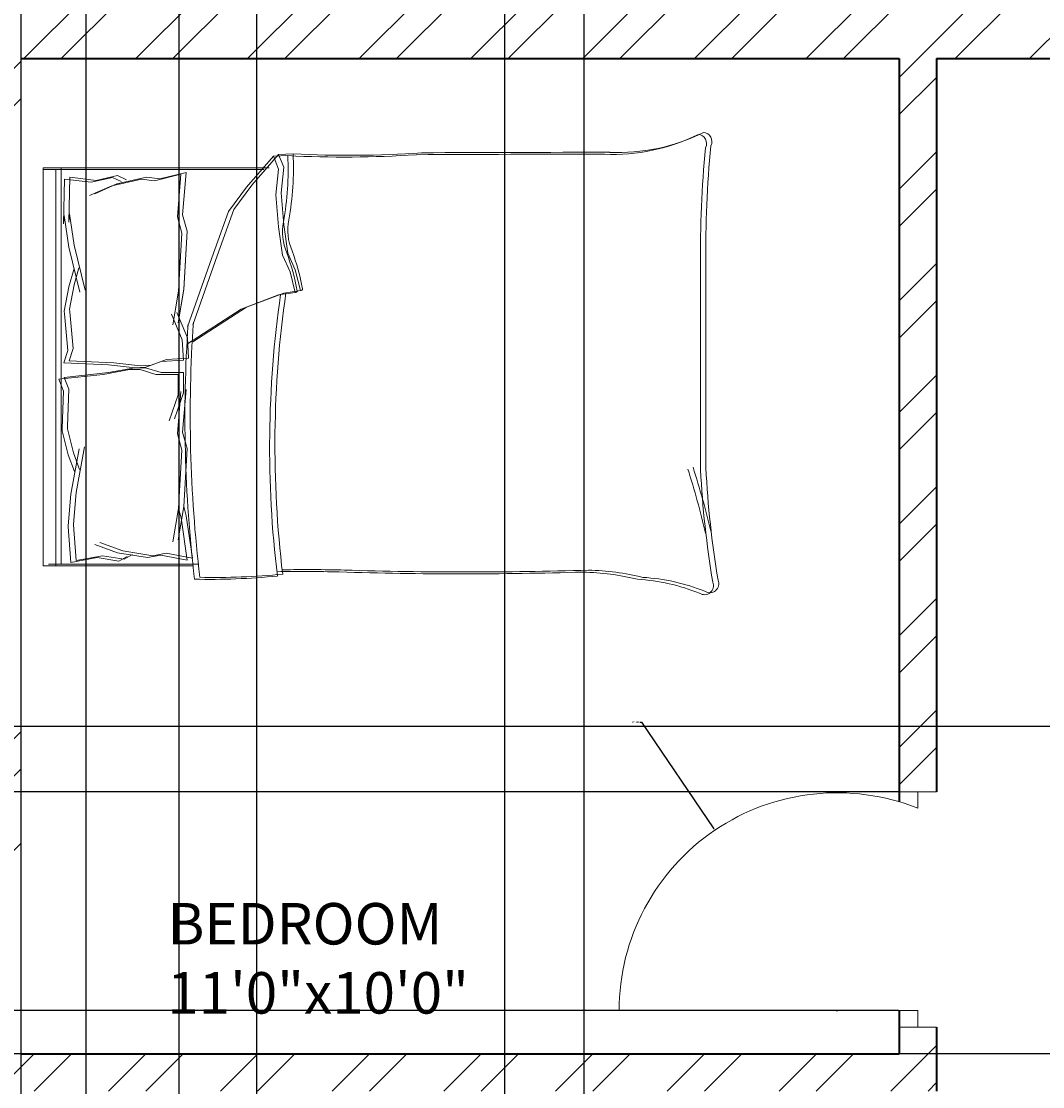
# Model space of a CAD drawing. Units: inches. Extents: x 1748 to 2382, y 1346 to 2284.
# Tile 5 of 26: x 1901 to 2024, y 1602 to 1730. Entities that reach past the tile are written whole.
import ezdxf

# ---------------------------------------------------------------- set-up
doc = ezdxf.new("R2010")
doc.units = ezdxf.units.IN
for name, color, linetype, lineweight in [('A-ANNO-DIMS', 2, 'Continuous', 18), ('A-AREA-IDEN', 7, 'Continuous', 18), ('A-DOOR', 21, 'Continuous', 18), ('A-FURN', 8, 'Continuous', 13), ('A-WALL', 7, 'Continuous', 35), ('A-WALL-PATT', 9, 'Continuous', 13)]:
    doc.layers.add(name, color=color, linetype=linetype, lineweight=lineweight)
doc.styles.get("Standard").update_dxf_attribs({"font": 'arial.ttf'})
doc.dimstyles.get("Standard").update_dxf_attribs({"dimtxt": 0.18, "dimasz": 0.18, "dimexe": 0.18, "dimexo": 0.0625, "dimgap": 0.09, "dimtad": 0, "dimtih": 1, "dimtoh": 1, "dimdec": 4, "dimzin": 0, "dimdsep": 46, "dimtxsty": 'Standard', "dimcen": 0.09, "dimadec": 0, "dimazin": 0, "dimtfac": 1, "dimtdec": 4, "dimtofl": 0, "dimtmove": 0, "dimatfit": 3, "dimfxl": 1, "dimtolj": 1, "dimtzin": 0, "dimarcsym": 0})

# ---------------------------------------------------------------- blocks, each defined once
blk = doc.blocks.new('BED-DOUBLE')
for p, q in [((3.48, 63.33), (3.48, 81.44)), ((3.48, 63.33), (3.48, 81.44)), ((3.48, 81.44), (51.49, 81.44)), ((51.27, 81.44), (51.27, 54.83)), ((51.27, 81.44), (51.27, 54.83)), ((51.49, 81.44), (51.49, 80.8)), ((3.48, 79.91), (51.27, 79.91)), ((3.48, 79.91), (51.27, 79.91)), ((3.7, 62.69), (3.7, 80.8)), ((3.7, 62.69), (3.7, 80.8)), ((51.49, 80.8), (51.49, 54.19)), ((51.49, 80.8), (51.49, 54.19)), ((3.7, 79.27), (51.49, 79.27)), ((3.7, 79.27), (51.49, 79.27)), ((3.9, 78.11), (8.18, 78.43)), ((3.9, 78.11), (8.18, 78.43)), ((8.18, 78.43), (8.29, 78.42)), ((8.18, 78.43), (8.28, 78.42)), ((8.28, 78.42), (12.11, 78.13)), ((8.29, 78.42), (12.11, 78.13)), ((14.86, 77.69), (16.88, 78.42)), ((14.86, 77.69), (16.88, 78.42)), ((16.88, 78.42), (19.77, 79.14)), ((16.88, 78.42), (19.77, 79.14)), ((17.11, 77.78), (20, 78.5)), ((17.11, 77.78), (20, 78.5)), ((19.77, 79.14), (20.09, 79.14)), ((19.77, 79.14), (20.09, 79.14)), ((20, 78.5), (20.32, 78.5)), ((20, 78.5), (20.32, 78.5)), ((20.09, 79.14), (24.54, 78.99)), ((20.09, 79.14), (24.54, 78.99)), ((20.32, 78.5), (24.77, 78.36)), ((20.32, 78.5), (24.77, 78.36)), ((24.54, 78.99), (25.98, 79.57)), ((24.54, 78.99), (25.98, 79.57)), ((24.77, 78.36), (26.21, 78.93)), ((24.77, 78.36), (26.21, 78.93)), ((25.98, 79.57), (26.56, 74.22)), ((25.98, 79.57), (26.56, 74.22)), ((26.21, 78.93), (26.79, 73.58)), ((26.21, 78.93), (26.79, 73.58)), ((27.98, 78.95), (27.73, 73.58)), ((27.98, 78.95), (27.73, 73.58)), ((29.46, 78.46), (27.98, 78.95)), ((29.46, 78.46), (27.98, 78.95)), ((33.88, 78.89), (29.46, 78.46)), ((33.88, 78.89), (29.46, 78.46)), ((34.21, 78.91), (33.88, 78.89)), ((34.2, 78.91), (33.88, 78.89)), ((37.14, 78.37), (34.2, 78.91)), ((37.14, 78.37), (34.21, 78.91)), ((41.91, 78.37), (36.5, 77.02)), ((41.91, 78.37), (36.5, 77.02)), ((45.71, 78.9), (41.91, 78.37)), ((45.71, 78.9), (41.91, 78.37)), ((50.11, 78.89), (44.71, 78.98)), ((44.71, 78.98), (45.71, 78.9)), ((50.11, 78.89), (44.71, 78.98)), ((44.71, 78.98), (45.71, 78.9)), ((50.11, 78.89), (49.73, 75.68)), ((50.11, 78.89), (49.73, 75.68)), ((3.89, 78.13), (4.47, 74.95)), ((3.9, 78.13), (4.47, 74.95)), ((4.12, 77.49), (4.7, 74.31)), ((4.12, 77.49), (4.7, 74.31)), ((4.13, 77.47), (8.41, 77.8)), ((4.13, 77.47), (8.41, 77.8)), ((8.41, 77.8), (8.51, 77.78)), ((8.41, 77.8), (8.51, 77.78)), ((8.51, 77.78), (12.34, 77.49)), ((8.51, 77.78), (12.34, 77.49)), ((12.11, 78.13), (17.6, 77.12)), ((12.11, 78.13), (17.6, 77.12)), ((12.34, 77.49), (17.83, 76.48)), ((12.34, 77.49), (17.83, 76.48)), ((15.08, 77.05), (17.11, 77.78)), ((15.08, 77.05), (17.11, 77.78)), ((28.21, 78.31), (27.96, 72.94)), ((28.21, 78.31), (27.96, 72.94)), ((29.68, 77.83), (28.21, 78.31)), ((29.68, 77.83), (28.21, 78.31)), ((34.11, 78.25), (29.68, 77.83)), ((34.11, 78.25), (29.68, 77.83)), ((34.43, 78.27), (34.11, 78.25)), ((34.43, 78.27), (34.11, 78.25)), ((37.36, 77.73), (34.43, 78.27)), ((37.36, 77.73), (34.43, 78.27)), ((42.14, 77.73), (36.72, 76.38)), ((42.14, 77.73), (36.72, 76.38)), ((39.2, 77.77), (37.14, 78.37)), ((39.2, 77.77), (37.14, 78.37)), ((39.43, 77.13), (37.36, 77.73)), ((39.43, 77.13), (37.36, 77.73)), ((45.94, 78.26), (42.14, 77.73)), ((45.94, 78.26), (42.14, 77.73)), ((50.34, 78.25), (44.94, 78.34)), ((44.94, 78.34), (45.94, 78.26)), ((50.34, 78.25), (44.94, 78.34)), ((44.94, 78.34), (45.94, 78.26)), ((50.34, 78.25), (49.96, 75.04)), ((50.34, 78.25), (49.96, 75.04)), ((49.31, 73.19), (48.13, 75.87)), ((49.31, 73.19), (48.13, 75.87)), ((4.47, 74.95), (4.04, 72.34)), ((4.47, 74.95), (4.04, 72.34)), ((5.05, 72.49), (6.06, 75.24)), ((5.05, 72.49), (6.06, 75.24)), ((5.28, 71.85), (6.29, 74.6)), ((5.28, 71.85), (6.29, 74.6)), ((49.54, 72.55), (48.36, 75.23)), ((49.54, 72.55), (48.36, 75.23)), ((49.73, 75.68), (50.33, 73.11)), ((49.73, 75.68), (50.33, 73.11)), ((49.96, 75.04), (50.56, 72.47)), ((49.96, 75.04), (50.56, 72.47)), ((4.7, 74.31), (4.27, 71.7)), ((4.7, 74.31), (4.27, 71.7)), ((26.56, 74.22), (27.14, 71.04)), ((26.56, 74.22), (27.14, 71.04)), ((26.79, 73.58), (27.37, 70.4)), ((26.79, 73.58), (27.37, 70.4)), ((27.73, 73.58), (27.35, 70.37)), ((27.73, 73.58), (27.36, 70.37)), ((4.04, 72.34), (4.62, 71.33)), ((4.04, 72.34), (4.62, 71.33)), ((4.47, 68.87), (5.05, 72.49)), ((4.47, 68.87), (5.05, 72.49)), ((27.96, 72.94), (27.58, 69.73)), ((27.96, 72.94), (27.58, 69.73)), ((50.11, 69.61), (49.31, 73.19)), ((50.11, 69.61), (49.31, 73.19)), ((50.34, 68.98), (49.54, 72.55)), ((50.34, 68.98), (49.54, 72.55)), ((50.33, 73.11), (49.81, 72.06)), ((50.33, 73.11), (49.81, 72.06)), ((50.56, 72.47), (50.04, 71.42)), ((50.56, 72.47), (50.04, 71.42)), ((4.27, 71.7), (4.85, 70.69)), ((4.27, 71.7), (4.85, 70.69)), ((4.7, 68.23), (5.28, 71.85)), ((4.7, 68.23), (5.28, 71.85)), ((27.14, 71.04), (27.14, 69.74)), ((27.14, 71.04), (27.14, 69.74)), ((27.14, 69.74), (26.56, 67.86)), ((27.14, 69.74), (26.56, 67.86)), ((27.35, 70.37), (27.44, 69.07)), ((27.36, 70.37), (27.44, 69.07)), ((27.37, 70.4), (27.37, 69.1)), ((27.37, 70.4), (27.37, 69.1)), ((27.58, 69.73), (27.66, 68.43)), ((27.58, 69.73), (27.66, 68.43)), ((49.92, 68.01), (50.11, 69.61)), ((49.92, 68.01), (50.11, 69.61)), ((4.76, 67.28), (4.47, 68.87)), ((4.76, 67.28), (4.47, 68.87)), ((4.99, 66.64), (4.7, 68.23)), ((4.99, 66.64), (4.7, 68.23)), ((27.37, 69.1), (26.79, 67.22)), ((27.37, 69.1), (26.79, 67.22)), ((27.44, 69.07), (28.13, 67.23)), ((27.44, 69.07), (28.13, 67.23)), ((27.66, 68.43), (28.36, 66.59)), ((27.66, 68.43), (28.36, 66.59)), ((50.15, 67.37), (50.34, 68.98)), ((50.15, 67.37), (50.34, 68.98)), ((4.18, 64.1), (4.76, 67.28)), ((4.18, 64.1), (4.76, 67.28)), ((26.56, 67.86), (26.56, 65.18)), ((26.56, 67.86), (26.56, 65.18)), ((26.79, 67.22), (26.79, 64.54)), ((26.79, 67.22), (26.79, 64.54)), ((28.13, 67.23), (28.3, 64.55)), ((28.13, 67.23), (28.3, 64.55)), ((50.7, 64.87), (49.92, 68.01)), ((50.7, 64.87), (49.92, 68.01)), ((50.93, 64.23), (50.15, 67.37)), ((50.93, 64.23), (50.15, 67.37)), ((4.41, 63.46), (4.99, 66.64)), ((4.41, 63.46), (4.99, 66.64)), ((6.38, 65.81), (10.41, 65.15)), ((6.38, 65.81), (10.41, 65.15)), ((24.1, 65.18), (20.96, 66.27)), ((24.1, 65.18), (20.96, 66.27)), ((24.33, 64.54), (21.19, 65.63)), ((24.33, 64.54), (21.19, 65.63)), ((28.36, 66.59), (28.53, 63.91)), ((28.36, 66.59), (28.53, 63.91)), ((30.75, 64.7), (33.82, 65.99)), ((30.75, 64.7), (33.82, 65.99)), ((32.56, 65.81), (36.6, 65.15)), ((32.56, 65.81), (36.6, 65.15)), ((9.28, 64.83), (4.18, 64.1)), ((9.28, 64.83), (4.18, 64.1)), ((6.61, 65.18), (10.64, 64.51)), ((6.61, 65.18), (10.64, 64.51)), ((10.41, 65.15), (9.28, 64.83)), ((10.41, 65.15), (9.28, 64.83)), ((10.64, 64.51), (9.51, 64.19)), ((10.64, 64.51), (9.51, 64.19)), ((10.41, 65.15), (17.42, 64.72)), ((10.41, 65.15), (17.42, 64.72)), ((10.64, 64.51), (17.65, 64.08)), ((10.64, 64.51), (17.65, 64.08)), ((17.42, 64.72), (19.38, 65.27)), ((17.42, 64.72), (19.38, 65.27)), ((17.65, 64.08), (19.61, 64.64)), ((17.65, 64.08), (19.61, 64.64)), ((19.38, 65.27), (24.52, 64.87)), ((19.38, 65.27), (24.52, 64.87)), ((19.61, 64.64), (24.74, 64.23)), ((19.61, 64.64), (24.74, 64.23)), ((26.56, 65.18), (24.1, 65.18)), ((26.56, 65.18), (24.1, 65.18)), ((26.79, 64.54), (24.33, 64.54)), ((26.79, 64.54), (24.33, 64.54)), ((28.3, 64.55), (30.75, 64.7)), ((28.3, 64.55), (30.75, 64.7)), ((30.98, 64.06), (34.05, 65.35)), ((30.98, 64.06), (34.05, 65.35)), ((32.79, 65.18), (36.83, 64.51)), ((32.79, 65.18), (36.82, 64.51)), ((36.6, 65.15), (43.61, 64.72)), ((36.6, 65.15), (43.61, 64.72)), ((36.82, 64.51), (43.83, 64.08)), ((36.83, 64.51), (43.83, 64.08)), ((43.61, 64.72), (45.57, 65.27)), ((43.61, 64.72), (45.57, 65.27)), ((43.83, 64.08), (45.8, 64.64)), ((43.83, 64.08), (45.79, 64.64)), ((45.57, 65.27), (50.7, 64.87)), ((45.57, 65.27), (50.7, 64.87)), ((45.79, 64.64), (50.93, 64.23)), ((45.8, 64.64), (50.93, 64.23)), ((9.51, 64.19), (4.41, 63.46)), ((9.51, 64.19), (4.41, 63.46)), ((28.53, 63.91), (30.98, 64.06)), ((28.53, 63.91), (30.98, 64.06)), ((30.26, 64.06), (34.45, 57.57)), ((30.26, 64.06), (34.45, 57.57)), ((30.49, 63.42), (34.68, 56.93)), ((30.49, 63.42), (34.68, 56.93)), ((40.64, 61.13), (32.31, 64.06)), ((40.64, 61.13), (32.31, 64.06)), ((40.87, 60.49), (32.53, 63.42)), ((40.87, 60.49), (32.53, 63.42)), ((46.22, 59.11), (40.64, 61.13)), ((46.22, 59.11), (40.64, 61.13)), ((46.45, 58.48), (40.87, 60.49)), ((46.45, 58.48), (40.87, 60.49)), ((49.16, 56.95), (46.22, 59.11)), ((49.16, 56.95), (46.22, 59.11)), ((49.39, 56.31), (46.45, 58.48)), ((49.39, 56.31), (46.45, 58.48)), ((34.45, 57.57), (36.15, 53.08)), ((34.45, 57.57), (36.15, 53.08)), ((34.68, 56.93), (36.38, 52.44)), ((34.68, 56.93), (36.38, 52.44)), ((52.87, 53.7), (49.16, 56.95)), ((52.87, 53.7), (49.16, 56.95)), ((53.1, 53.06), (49.39, 56.31)), ((53.1, 53.06), (49.39, 56.31)), ((36.15, 53.08), (36.46, 51.07)), ((36.15, 53.08), (36.46, 51.07)), ((40.95, 52.61), (44.36, 53.08)), ((40.95, 52.61), (44.36, 53.08)), ((44.36, 53.08), (48.23, 53.39)), ((44.36, 53.08), (48.23, 53.39)), ((44.59, 52.44), (48.46, 52.75)), ((44.59, 52.44), (48.46, 52.75)), ((48.23, 53.39), (51.33, 53.08)), ((48.23, 53.39), (51.33, 53.08)), ((48.46, 52.75), (51.56, 52.44)), ((48.46, 52.75), (51.56, 52.44)), ((51.33, 53.08), (52.87, 53.7)), ((51.33, 53.08), (52.87, 53.7)), ((51.56, 52.44), (53.1, 53.06)), ((51.56, 52.44), (53.1, 53.06)), ((52.95, 51.95), (52.87, 53.7, 3.87)), ((52.95, 51.95), (52.87, 53.7, 3.87)), ((53.18, 51.31), (53.1, 53.06, 3.87)), ((53.18, 51.31), (53.1, 53.06, 3.87)), ((36.38, 52.44), (36.69, 50.43)), ((36.38, 52.44), (36.69, 50.43)), ((36.46, 51.07), (38.94, 51.69)), ((36.46, 51.07), (38.94, 51.69)), ((38.94, 51.69), (40.95, 52.61)), ((38.94, 51.69), (40.95, 52.61)), ((39.17, 51.05), (41.18, 51.97)), ((39.17, 51.05), (41.18, 51.97)), ((41.18, 51.97), (44.59, 52.44)), ((41.18, 51.97), (44.59, 52.44)), ((36.69, 50.43), (39.17, 51.05)), ((36.69, 50.43), (39.17, 51.05)), ((15.06, 2.2), (39.68, 2.2)), ((15.06, 2.2), (39.68, 2.2)), ((15.29, 1.56), (39.91, 1.56)), ((15.29, 1.56), (39.91, 1.56))]:
    blk.add_line(p, q)
for centre, radius, start, end in [((21.36, -100.61), 164.97, 86.0865, 96.7821), ((21.36, -100.61), 164.97, 86.0865, 96.7821), ((85.16, 61.35), 83.31, 178.7218, 185.604), ((85.16, 61.35), 83.31, 178.7218, 185.604), ((21.59, -101.25), 164.97, 86.0865, 96.7821), ((21.59, -101.25), 164.97, 86.0865, 96.7821), ((85.39, 60.71), 83.31, 178.7218, 185.604), ((85.39, 60.71), 83.31, 178.7218, 185.604), ((17.76, -74.87), 129.02, 81.7845, 96.9006), ((17.76, -74.87), 129.02, 81.7845, 96.9006), ((17.98, -75.51), 129.02, 81.7845, 96.9006), ((17.98, -75.51), 129.02, 81.7845, 96.9006), ((-167.31, 50.27), 170.11, 358.4762, 1.0082), ((-167.31, 50.27), 170.11, 358.4762, 1.0082), ((-167.08, 49.63), 170.11, 358.4762, 1.0082), ((-167.08, 49.63), 170.11, 358.4762, 1.0082), ((31.15, 79.96), 29.65, 280.6617, 289.8806), ((31.15, 79.96), 29.65, 280.6617, 289.8806), ((31.38, 79.32), 29.65, 280.6617, 289.8806), ((31.38, 79.32), 29.65, 280.6617, 289.8806), ((43.74, 46.38), 6.22, 78.6608, 113.7384), ((43.74, 46.38), 6.22, 78.6608, 113.7384), ((43.97, 45.74), 6.22, 78.6608, 113.7384), ((43.97, 45.74), 6.22, 78.6608, 113.7384), ((51.33, 88.1), 36.18, 259.8763, 272.5657), ((51.33, 88.1), 36.18, 259.8763, 272.5657), ((51.56, 87.46), 36.18, 259.8763, 272.5657), ((51.56, 87.46), 36.18, 259.8763, 272.5657), ((182.27, 45.13), 129.5, 176.9791, 183.8365), ((182.27, 45.13), 129.5, 176.9791, 183.8365), ((36.64, 51), 0.185, 160.2464, 271.1377), ((36.64, 51), 0.185, 160.2464, 271.1377), ((36.87, 50.36), 0.185, 160.2464, 271.1377), ((36.86, 50.36), 0.185, 160.2464, 271.1377), ((182.49, 44.49), 129.5, 176.9791, 183.8365), ((182.49, 44.49), 129.5, 176.9791, 183.8365), ((484.82, 30.83), 482.31, 178.2277, 181.7185), ((484.82, 30.83), 482.31, 178.2277, 181.7185), ((485.05, 30.19), 482.31, 178.2277, 181.7185), ((485.05, 30.19), 482.31, 178.2277, 181.7185), ((-4508.74, 13.62), 4561.86, 0.00217, 0.28689), ((-4508.74, 13.62), 4561.86, 0.00217, 0.28689), ((-4508.51, 12.98), 4561.86, 0.00217, 0.28689), ((-4508.51, 12.98), 4561.86, 0.00217, 0.28689), ((-26.9, 16.93), 29.63, 346.0648, 358.9113), ((-26.9, 16.93), 29.63, 346.0648, 358.9113), ((-26.67, 16.29), 29.63, 346.0648, 358.9113), ((-26.67, 16.29), 29.63, 346.0648, 358.9113), ((76.16, 12.78), 23.07, 177.4714, 206.4681), ((76.16, 12.78), 23.07, 177.4714, 206.4681), ((76.39, 12.14), 23.07, 177.4714, 206.4681), ((76.39, 12.14), 23.07, 177.4714, 206.4681), ((-21.66, 11.17), 23.56, 337.9751, 356.652), ((-21.66, 11.17), 23.56, 337.9751, 356.652), ((-21.43, 10.53), 23.56, 337.9751, 356.652), ((-21.43, 10.53), 23.56, 337.9751, 356.652), ((-17.22, 105.16), 106.46, 283.3832, 287.7053), ((-17.22, 105.16), 106.46, 283.3832, 287.7053), ((-16.99, 104.52), 106.46, 283.3832, 287.7053), ((-16.99, 104.52), 106.46, 283.3832, 287.7053), ((1.09, 1.73), 1.09, 146.1736, 293.4781), ((1.09, 1.73), 1.09, 146.1736, 293.4781), ((1.32, 1.09), 1.09, 146.1736, 293.4781), ((1.32, 1.09), 1.09, 146.1736, 293.4781), ((21.43, -119.39), 121.76, 92.9958, 99.4091), ((21.43, -119.39), 121.76, 92.9958, 99.4091), ((21.66, -120.03), 121.76, 92.9958, 99.4091), ((21.66, -120.03), 121.76, 92.9958, 99.4091), ((41.15, -130.83), 133.04, 84.4998, 90.6351), ((41.15, -130.83), 133.04, 84.4998, 90.6351), ((41.38, -131.47), 133.04, 84.4998, 90.6351), ((41.38, -131.47), 133.04, 84.4998, 90.6351), ((54.41, 2.57), 1.1, 242.6588, 356.02), ((54.41, 2.57), 1.1, 242.6588, 356.02), ((54.64, 1.93), 1.1, 242.6588, 356.02), ((54.64, 1.93), 1.1, 242.6588, 356.02)]:
    blk.add_arc(centre, radius, start, end)
blk = doc.blocks.new('*D50')
at = {"layer": 'A-ANNO-DIMS', "color": 0, "lineweight": -2, "transparency": 16777216}
for p, q in [((1869.96, 2223.79), (1869.96, 1360.47)), ((1908.44, 2223.79), (1908.44, 1360.47)), ((1870.14, 1360.65), (1888.81, 1360.65)), ((1908.26, 1360.65), (1889.6, 1360.65))]:
    blk.add_line(p, q, dxfattribs=at)
at = {"layer": 'A-ANNO-DIMS', "color": 0, "transparency": 16777216}
for points in [[(1870.14, 1360.68), (1870.14, 1360.62), (1869.96, 1360.65)], [(1908.26, 1360.68), (1908.26, 1360.62), (1908.44, 1360.65)]]:
    blk.add_solid(points, dxfattribs=at)
at = {"layer": 'Defpoints', "color": 0, "transparency": 16777216}
for p in [(1869.96, 2223.85), (1908.44, 2223.85), (1908.44, 1360.65)]:
    blk.add_point(p, dxfattribs=at)
at = {"layer": 'A-ANNO-DIMS', "color": 0, "transparency": 16777216, "insert": (1889.2, 1360.65), "char_height": 0.18, "attachment_point": 5}
blk.add_mtext('\\A1;38.48', dxfattribs=at)
blk = doc.blocks.new('*D51')
at = {"layer": 'A-ANNO-DIMS', "color": 0, "lineweight": -2, "transparency": 16777216}
for p, q in [((1968.44, 2223.79), (1968.44, 1360.47)), ((2040.07, 2223.79), (2040.07, 1360.47)), ((1968.62, 1360.65), (2003.86, 1360.65)), ((2039.89, 1360.65), (2004.65, 1360.65))]:
    blk.add_line(p, q, dxfattribs=at)
at = {"layer": 'A-ANNO-DIMS', "color": 0, "transparency": 16777216}
for points in [[(1968.62, 1360.68), (1968.62, 1360.62), (1968.44, 1360.65)], [(2039.89, 1360.68), (2039.89, 1360.62), (2040.07, 1360.65)]]:
    blk.add_solid(points, dxfattribs=at)
at = {"layer": 'Defpoints', "color": 0, "transparency": 16777216}
for p in [(1968.44, 2223.85), (2040.07, 2223.85), (2040.07, 1360.65)]:
    blk.add_point(p, dxfattribs=at)
at = {"layer": 'A-ANNO-DIMS', "color": 0, "transparency": 16777216, "insert": (2004.26, 1360.65), "char_height": 0.18, "attachment_point": 5}
blk.add_mtext('\\A1;71.62', dxfattribs=at)
blk = doc.blocks.new('*D55')
at = {"layer": 'A-ANNO-DIMS', "color": 0, "lineweight": -2, "transparency": 16777216}
for p, q in [((2288.4, 1645.3), (1779.88, 1645.3)), ((1780.06, 1645.12), (1780.06, 1625.76)), ((1780.06, 1606.03), (1780.06, 1625.39)), ((2288.4, 1605.85), (1779.88, 1605.85))]:
    blk.add_line(p, q, dxfattribs=at)
at = {"layer": 'A-ANNO-DIMS', "color": 0, "transparency": 16777216}
for points in [[(1780.03, 1645.12), (1780.09, 1645.12), (1780.06, 1645.3)], [(1780.03, 1606.03), (1780.09, 1606.03), (1780.06, 1605.85)]]:
    blk.add_solid(points, dxfattribs=at)
at = {"layer": 'Defpoints', "color": 0, "transparency": 16777216}
for p in [(1780.06, 1645.3), (2288.46, 1645.3), (2288.46, 1605.85)]:
    blk.add_point(p, dxfattribs=at)
at = {"layer": 'A-ANNO-DIMS', "color": 0, "transparency": 16777216, "insert": (1780.06, 1625.58), "char_height": 0.18, "attachment_point": 5}
blk.add_mtext('\\A1;39.454', dxfattribs=at)
blk = doc.blocks.new('*D64')
at = {"layer": 'A-ANNO-DIMS', "color": 0, "lineweight": -2, "transparency": 16777216}
for p, q in [((1900.64, 1476.91), (1900.64, 2274.93)), ((1900.82, 2274.75), (1909.7, 2274.75)), ((1919.5, 2274.75), (1910.62, 2274.75)), ((1919.68, 1476.91), (1919.68, 2274.93))]:
    blk.add_line(p, q, dxfattribs=at)
at = {"layer": 'A-ANNO-DIMS', "color": 0, "transparency": 16777216}
for points in [[(1900.82, 2274.78), (1900.82, 2274.72), (1900.64, 2274.75)], [(1919.5, 2274.78), (1919.5, 2274.72), (1919.68, 2274.75)]]:
    blk.add_solid(points, dxfattribs=at)
at = {"layer": 'Defpoints', "color": 0, "transparency": 16777216}
for p in [(1919.68, 2274.75), (1900.64, 1476.85), (1919.68, 1476.85)]:
    blk.add_point(p, dxfattribs=at)
at = {"layer": 'A-ANNO-DIMS', "color": 0, "transparency": 16777216, "insert": (1910.16, 2274.75), "char_height": 0.18, "attachment_point": 5}
blk.add_mtext('\\A1;19.035', dxfattribs=at)
blk = doc.blocks.new('*D74')
at = {"layer": 'A-ANNO-DIMS', "color": 0, "lineweight": -2, "transparency": 16777216}
for p, q in [((2006.4, 1637.45), (1779.88, 1637.45)), ((1780.06, 1637.27), (1780.06, 1624.43)), ((1780.06, 1611.24), (1780.06, 1624.07)), ((2006.4, 1611.06), (1779.88, 1611.06))]:
    blk.add_line(p, q, dxfattribs=at)
at = {"layer": 'A-ANNO-DIMS', "color": 0, "transparency": 16777216}
for points in [[(1780.03, 1637.27), (1780.09, 1637.27), (1780.06, 1637.45)], [(1780.03, 1611.24), (1780.09, 1611.24), (1780.06, 1611.06)]]:
    blk.add_solid(points, dxfattribs=at)
at = {"layer": 'Defpoints', "color": 0, "transparency": 16777216}
for p in [(1780.06, 1637.45), (2006.46, 1637.45), (2006.46, 1611.06)]:
    blk.add_point(p, dxfattribs=at)
at = {"layer": 'A-ANNO-DIMS', "color": 0, "transparency": 16777216, "insert": (1780.06, 1624.25), "char_height": 0.18, "attachment_point": 5}
blk.add_mtext('\\A1;26.39', dxfattribs=at)
blk = doc.blocks.new('*D79')
at = {"layer": 'A-ANNO-DIMS', "color": 0, "lineweight": -2, "transparency": 16777216}
for p, q in [((1929, 1854.79), (1929, 1360.47)), ((1958.9, 1854.79), (1958.9, 1360.47)), ((1929.18, 1360.65), (1943.62, 1360.65)), ((1958.72, 1360.65), (1944.27, 1360.65))]:
    blk.add_line(p, q, dxfattribs=at)
at = {"layer": 'A-ANNO-DIMS', "color": 0, "transparency": 16777216}
for points in [[(1929.18, 1360.68), (1929.18, 1360.62), (1929, 1360.65)], [(1958.72, 1360.68), (1958.72, 1360.62), (1958.9, 1360.65)]]:
    blk.add_solid(points, dxfattribs=at)
at = {"layer": 'Defpoints', "color": 0, "transparency": 16777216}
for p in [(1929, 1854.85), (1958.9, 1854.85), (1958.9, 1360.65)]:
    blk.add_point(p, dxfattribs=at)
at = {"layer": 'A-ANNO-DIMS', "color": 0, "transparency": 16777216, "insert": (1943.95, 1360.65), "char_height": 0.18, "attachment_point": 5}
blk.add_mtext('\\A1;29.9', dxfattribs=at)
blk = doc.blocks.new('*D85')
at = {"layer": 'A-ANNO-DIMS', "color": 0, "lineweight": -2, "transparency": 16777216}
for p, q in [((1975.22, 1645.84), (1975.4, 1645.84)), ((1975.4, 1645.84), (1984.14, 1632.95)), ((1998.97, 1610.97), (1998.97, 1611.15)), ((1998.88, 1611.06), (1999.06, 1611.06))]:
    blk.add_line(p, q, dxfattribs=at)
at = {"layer": 'A-ANNO-DIMS', "color": 0, "transparency": 16777216}
blk.add_solid([(1984.17, 1632.96), (1984.12, 1632.93), (1984.24, 1632.8)], dxfattribs=at)
at = {"layer": 'Defpoints', "color": 0, "transparency": 16777216}
for p in [(1984.24, 1632.8), (1998.97, 1611.06)]:
    blk.add_point(p, dxfattribs=at)
at = {"layer": 'A-ANNO-DIMS', "color": 0, "transparency": 16777216, "insert": (1974.67, 1645.84), "char_height": 0.18, "attachment_point": 5}
blk.add_mtext('\\A1;R26.263', dxfattribs=at)

msp = doc.modelspace()

# ---------------------------------------------------------------- hatches: boundary and pattern name
at = {"layer": 'A-WALL-PATT'}
h = msp.add_hatch(dxfattribs=at)
h.set_pattern_fill('ANSI32', color=256)
h.paths.add_polyline_path([(1908.4445, 2232.8497), (1821.9607, 2232.8497), (1821.9607, 2223.8497), (1865.4607, 2223.8497), (1865.4607, 2209.9185), (1869.9607, 2209.9185), (1869.9607, 2223.8497), (1908.4445, 2223.8497), (1908.4445, 2228.3497)])
h.paths.add_polyline_path([(2040.0683, 2232.8497), (1968.4445, 2232.8497), (1968.4445, 2223.8497), (2025.9607, 2223.8497), (2025.9607, 2130.3497), (2032.1341, 2130.3497), (2032.1341, 2132.5997), (2032.1341, 2134.8497), (2030.4607, 2134.8497), (2030.4607, 2223.8497), (2040.0683, 2223.8497)])
h.paths.add_polyline_path([(2091.3969, 2232.8497), (2064.0683, 2232.8497), (2064.0683, 2223.8497), (2078.4607, 2223.8497), (2078.4607, 2134.8497), (2051.1563, 2134.8497), (2051.1563, 2130.3497), (2078.4607, 2130.3497), (2078.4607, 2128.6813), (2082.9607, 2128.6813), (2082.9607, 2130.3497), (2086.1879, 2130.3497), (2086.1879, 2132.5997), (2086.1879, 2134.8497), (2082.9607, 2134.8497), (2082.9607, 2223.8497), (2091.3969, 2223.8497), (2091.3969, 2228.3497)])
h.paths.add_polyline_path([(2167.0164, 2232.8497), (2115.3969, 2232.8497), (2115.3969, 2223.8497), (2130.9607, 2223.8497), (2130.9607, 2134.8497), (2106.9607, 2134.8497), (2106.9607, 2130.3497), (2135.4607, 2130.3497), (2135.4607, 2223.8497), (2167.0164, 2223.8497), (2167.0164, 2228.3497)])
h.paths.add_polyline_path([(1869.9607, 2149.9185), (1865.4607, 2149.9185), (1865.4607, 2127.8942), (1869.9607, 2127.8942)])
h.paths.add_polyline_path([(2082.9607, 2104.4871), (2080.7107, 2104.4871), (2078.4607, 2104.4871), (2078.4607, 2103.8497), (1869.9607, 2103.8497), (1869.9607, 2108.6062), (1867.7107, 2108.6062), (1865.4607, 2108.6062), (1865.4607, 2103.8497), (1821.9607, 2103.8497), (1821.9607, 2099.3497), (1865.4607, 2099.3497), (1865.4607, 2094.7509), (1869.9607, 2094.7509), (1869.9607, 2099.3497), (2025.9607, 2099.3497), (2025.9607, 2096.4326), (2030.4607, 2096.4326), (2030.4607, 2099.3497), (2082.9607, 2099.3497)])
h.paths.add_polyline_path([(1928.9457, 1401.1212), (2176.8693, 1401.1212), (2176.8693, 1438.214), (1928.9457, 1438.214)], flags=9)
h.paths.add_polyline_path([(2122.2668, 2048.1927), (2177.9387, 2048.1927), (2177.9387, 2066.85), (2122.2668, 2066.85)], flags=9)
h.paths.add_polyline_path([(2272.688, 2153.8197), (2272.688, 2216.746), (2262.3845, 2216.746), (2262.3845, 2153.8197)], flags=9)
h.paths.add_polyline_path([(2157.2928, 2166.5593), (2196.3822, 2166.5593), (2196.3822, 2185.2167), (2157.2928, 2185.2167)], flags=9)
h.paths.add_polyline_path([(2089.3407, 2162.0698), (2124.3987, 2162.0698), (2124.3987, 2180.7272), (2089.3407, 2180.7272)], flags=9)
h.paths.add_polyline_path([(2037.4521, 2160.0913), (2072.5101, 2160.0913), (2072.5101, 2178.7486), (2037.4521, 2178.7486)], flags=9)
h.paths.add_polyline_path([(1884.7894, 2104.1554), (1923.6297, 2104.1554), (1923.6297, 2122.8127), (1884.7894, 2122.8127)], flags=9)
h.paths.add_polyline_path([(1851.2832, 2142.9749), (1851.2832, 2199.3051), (1840.9796, 2199.3051), (1840.9796, 2142.9749)], flags=9)
h.paths.add_polyline_path([(1844.8763, 2017.2834), (1844.8763, 2073.6136), (1834.5728, 2073.6136), (1834.5728, 2017.2834)], flags=9)
h.paths.add_polyline_path([(1897.1577, 2073.1279), (1935.9981, 2073.1279), (1935.9981, 2091.7853), (1897.1577, 2091.7853)], flags=9)
h.paths.add_polyline_path([(1952.3395, 1802.4231), (2008.0114, 1802.4231), (2008.0114, 1821.0805), (1952.3395, 1821.0805)], flags=9)
h.paths.add_polyline_path([(1978.8184, 1857.6841), (2017.7338, 1857.6841), (2017.7338, 1876.3415), (1978.8184, 1876.3415)], flags=9)
h.paths.add_polyline_path([(1979.6513, 1925.9516), (2008.8089, 1925.9516), (2008.8089, 1944.6089), (1979.6513, 1944.6089)], flags=9)
h.paths.add_polyline_path([(1838.5553, 1860.3527), (1877.3957, 1860.3527), (1877.3957, 1879.01), (1838.5553, 1879.01)], flags=9)
h.paths.add_polyline_path([(1883.9018, 1787.3013), (1883.9018, 1843.6315), (1873.5983, 1843.6315), (1873.5983, 1787.3013)], flags=9)
h.paths.add_polyline_path([(1873.7079, 1509.1938), (1873.7079, 1583.7709), (1863.4044, 1583.7709), (1863.4044, 1509.1938)], flags=9)
h.paths.add_polyline_path([(1916.2259, 1603.3681), (1955.0663, 1603.3681), (1955.0663, 1622.0254), (1916.2259, 1622.0254)], flags=9)
h.paths.add_polyline_path([(1876.3013, 1636.757), (1876.3013, 1693.0871), (1865.9978, 1693.0871), (1865.9978, 1636.757)], flags=9)
h.paths.add_polyline_path([(1921.3138, 1521.8316), (1964.0662, 1521.8316), (1964.0662, 1540.489), (1921.3138, 1540.489)], flags=9)
h.paths.add_polyline_path([(2017.5657, 1497.5078), (2046.7983, 1497.5078), (2046.7983, 1516.1651), (2017.5657, 1516.1651)], flags=9)
h.paths.add_polyline_path([(2066.8661, 1499.3902), (2096.0988, 1499.3902), (2096.0988, 1518.0475), (2066.8661, 1518.0475)], flags=9)
h.paths.add_polyline_path([(2155.4835, 1571.6596), (2198.2358, 1571.6596), (2198.2358, 1590.3169), (2155.4835, 1590.3169)], flags=9)
h.paths.add_polyline_path([(2094.9136, 1664.6812), (2150.5855, 1664.6812), (2150.5855, 1683.3386), (2094.9136, 1683.3386)], flags=9)
h.paths.add_polyline_path([(2257.6902, 1863.1628), (2269.8935, 1863.1628), (2269.8935, 1873.4664), (2257.6902, 1873.4664)], flags=9)
h.paths.add_polyline_path([(2164.0748, 1880.3089), (2189.8694, 1880.3089), (2189.8694, 1890.6124), (2164.0748, 1890.6124)], flags=9)
h.paths.add_polyline_path([(2239.4394, 1931.0585), (2268.8187, 1931.0585), (2268.8187, 1949.7159), (2239.4394, 1949.7159)], flags=9)
h = msp.add_hatch(dxfattribs=at)
h.set_pattern_fill('ANSI32', color=256)
h.paths.add_polyline_path([(2297.4607, 2232.8497), (2203.0164, 2232.8497), (2203.0164, 2223.8497), (2244.9607, 2223.8497), (2244.9607, 2127.8554), (2249.4607, 2127.8554), (2249.4607, 2223.8497), (2297.4607, 2223.8497)])
h.paths.add_polyline_path([(2297.4607, 2103.8497), (2249.4607, 2103.8497), (2249.4607, 2106.7497), (2247.2107, 2106.7497), (2244.9607, 2106.7497), (2244.9607, 2103.8497), (2130.9607, 2103.8497), (2130.9607, 2099.3497), (2288.4607, 2099.3497), (2288.4607, 2077.2008), (2297.4607, 2077.2008)])
h.paths.add_polyline_path([(1928.9457, 1401.1212), (2176.8693, 1401.1212), (2176.8693, 1438.214), (1928.9457, 1438.214)], flags=9)
h.paths.add_polyline_path([(2122.2668, 2048.1927), (2177.9387, 2048.1927), (2177.9387, 2066.85), (2122.2668, 2066.85)], flags=9)
h.paths.add_polyline_path([(2272.688, 2153.8197), (2272.688, 2216.746), (2262.3845, 2216.746), (2262.3845, 2153.8197)], flags=25)
h.paths.add_polyline_path([(2157.2928, 2166.5593), (2196.3822, 2166.5593), (2196.3822, 2185.2167), (2157.2928, 2185.2167)], flags=9)
h.paths.add_polyline_path([(2089.3407, 2162.0698), (2124.3987, 2162.0698), (2124.3987, 2180.7272), (2089.3407, 2180.7272)], flags=9)
h.paths.add_polyline_path([(2037.4521, 2160.0913), (2072.5101, 2160.0913), (2072.5101, 2178.7486), (2037.4521, 2178.7486)], flags=9)
h.paths.add_polyline_path([(1884.7894, 2104.1554), (1923.6297, 2104.1554), (1923.6297, 2122.8127), (1884.7894, 2122.8127)], flags=9)
h.paths.add_polyline_path([(1851.2832, 2142.9749), (1851.2832, 2199.3051), (1840.9796, 2199.3051), (1840.9796, 2142.9749)], flags=9)
h.paths.add_polyline_path([(1844.8763, 2017.2834), (1844.8763, 2073.6136), (1834.5728, 2073.6136), (1834.5728, 2017.2834)], flags=9)
h.paths.add_polyline_path([(1897.1577, 2073.1279), (1935.9981, 2073.1279), (1935.9981, 2091.7853), (1897.1577, 2091.7853)], flags=9)
h.paths.add_polyline_path([(1952.3395, 1802.4231), (2008.0114, 1802.4231), (2008.0114, 1821.0805), (1952.3395, 1821.0805)], flags=9)
h.paths.add_polyline_path([(1978.8184, 1857.6841), (2017.7338, 1857.6841), (2017.7338, 1876.3415), (1978.8184, 1876.3415)], flags=9)
h.paths.add_polyline_path([(1979.6513, 1925.9516), (2008.8089, 1925.9516), (2008.8089, 1944.6089), (1979.6513, 1944.6089)], flags=9)
h.paths.add_polyline_path([(1838.5553, 1860.3527), (1877.3957, 1860.3527), (1877.3957, 1879.01), (1838.5553, 1879.01)], flags=9)
h.paths.add_polyline_path([(1883.9018, 1787.3013), (1883.9018, 1843.6315), (1873.5983, 1843.6315), (1873.5983, 1787.3013)], flags=9)
h.paths.add_polyline_path([(1873.7079, 1509.1938), (1873.7079, 1583.7709), (1863.4044, 1583.7709), (1863.4044, 1509.1938)], flags=9)
h.paths.add_polyline_path([(1916.2259, 1603.3681), (1955.0663, 1603.3681), (1955.0663, 1622.0254), (1916.2259, 1622.0254)], flags=9)
h.paths.add_polyline_path([(1876.3013, 1636.757), (1876.3013, 1693.0871), (1865.9978, 1693.0871), (1865.9978, 1636.757)], flags=9)
h.paths.add_polyline_path([(1921.3138, 1521.8316), (1964.0662, 1521.8316), (1964.0662, 1540.489), (1921.3138, 1540.489)], flags=9)
h.paths.add_polyline_path([(2017.5657, 1497.5078), (2046.7983, 1497.5078), (2046.7983, 1516.1651), (2017.5657, 1516.1651)], flags=9)
h.paths.add_polyline_path([(2066.8661, 1499.3902), (2096.0988, 1499.3902), (2096.0988, 1518.0475), (2066.8661, 1518.0475)], flags=9)
h.paths.add_polyline_path([(2155.4835, 1571.6596), (2198.2358, 1571.6596), (2198.2358, 1590.3169), (2155.4835, 1590.3169)], flags=9)
h.paths.add_polyline_path([(2094.9136, 1664.6812), (2150.5855, 1664.6812), (2150.5855, 1683.3386), (2094.9136, 1683.3386)], flags=9)
h.paths.add_polyline_path([(2257.6902, 1863.1628), (2269.8935, 1863.1628), (2269.8935, 1873.4664), (2257.6902, 1873.4664)], flags=9)
h.paths.add_polyline_path([(2164.0748, 1880.3089), (2189.8694, 1880.3089), (2189.8694, 1890.6124), (2164.0748, 1890.6124)], flags=9)
h.paths.add_polyline_path([(2239.4394, 1931.0585), (2268.8187, 1931.0585), (2268.8187, 1949.7159), (2239.4394, 1949.7159)], flags=9)
h = msp.add_hatch(dxfattribs=at)
h.set_pattern_fill('ANSI32', color=256)
h.paths.add_polyline_path([(1919.6777, 1476.8497), (1900.6426, 1476.8497), (1900.6426, 1522.0826), (1898.3926, 1522.0826), (1896.1426, 1522.0826), (1896.1426, 1476.8497), (1857.1426, 1476.8497), (1857.1426, 1467.8497), (1896.1426, 1467.8497), (1919.6777, 1467.8497), (1919.6777, 1472.3497)])
h.paths.add_polyline_path([(2018.7873, 1472.3497), (2018.7873, 1476.8497), (2010.9607, 1476.8497), (2010.9607, 1560.8497), (2034.9607, 1560.8497), (2034.9607, 1565.3497), (2006.4607, 1565.3497), (2006.4607, 1476.8497), (1955.6777, 1476.8497), (1955.6777, 1467.8497), (2018.7873, 1467.8497)])
h.paths.add_polyline_path([(2152.3354, 1472.3497), (2152.3354, 1476.8497), (2115.9607, 1476.8497), (2115.9607, 1565.3497), (2109.2204, 1565.3497), (2109.2204, 1563.0997), (2109.2204, 1560.8497), (2111.4607, 1560.8497), (2111.4607, 1476.8497), (2095.3617, 1476.8497), (2095.3617, 1467.8497), (2152.3354, 1467.8497)])
h.paths.add_polyline_path([(2071.3617, 1476.8497), (2063.4607, 1476.8497), (2063.4607, 1560.8497), (2090.1865, 1560.8497), (2090.1865, 1565.3497), (2063.4607, 1565.3497), (2063.4607, 1572.5485), (2061.2107, 1572.5485), (2058.9607, 1572.5485), (2058.9607, 1565.3497), (2055.6281, 1565.3497), (2055.6281, 1560.8497), (2058.9607, 1560.8497), (2058.9607, 1476.8497), (2042.7873, 1476.8497), (2042.7873, 1467.8497), (2071.3617, 1467.8497), (2071.3617, 1472.3497)])
h.paths.add_polyline_path([(2297.4607, 1506.5652), (2288.4607, 1506.5652), (2288.4607, 1476.8497), (2212.3354, 1476.8497), (2212.3354, 1467.8497), (2297.4607, 1467.8497)])
h.paths.add_polyline_path([(2297.4607, 1645.3038), (2288.4607, 1645.3038), (2288.4607, 1605.8497), (2058.9607, 1605.8497), (2058.9607, 1600.1857), (2061.2107, 1600.1857), (2063.4607, 1600.1857), (2063.4607, 1601.3497), (2288.4607, 1601.3497), (2288.4607, 1566.5652), (2297.4607, 1566.5652)])
h.paths.add_polyline_path([(2010.9607, 1609.0561), (2008.7107, 1609.0561), (2006.4607, 1609.0561), (2006.4607, 1605.8497), (1900.6426, 1605.8497), (1900.6426, 1609.7171), (1898.3926, 1609.7171), (1896.1426, 1609.7171), (1896.1426, 1605.8497), (1857.1426, 1605.8497), (1857.1426, 1601.3497), (1896.1426, 1601.3497), (1896.1426, 1542.5447), (1900.6426, 1542.5447), (1900.6426, 1601.3497), (2010.9607, 1601.3497)])
h.paths.add_polyline_path([(1928.9457, 1401.1212), (2176.8693, 1401.1212), (2176.8693, 1438.214), (1928.9457, 1438.214)], flags=9)
h.paths.add_polyline_path([(2122.2668, 2048.1927), (2177.9387, 2048.1927), (2177.9387, 2066.85), (2122.2668, 2066.85)], flags=9)
h.paths.add_polyline_path([(2272.688, 2153.8197), (2272.688, 2216.746), (2262.3845, 2216.746), (2262.3845, 2153.8197)], flags=9)
h.paths.add_polyline_path([(2157.2928, 2166.5593), (2196.3822, 2166.5593), (2196.3822, 2185.2167), (2157.2928, 2185.2167)], flags=9)
h.paths.add_polyline_path([(2089.3407, 2162.0698), (2124.3987, 2162.0698), (2124.3987, 2180.7272), (2089.3407, 2180.7272)], flags=9)
h.paths.add_polyline_path([(2037.4521, 2160.0913), (2072.5101, 2160.0913), (2072.5101, 2178.7486), (2037.4521, 2178.7486)], flags=9)
h.paths.add_polyline_path([(1884.7894, 2104.1554), (1923.6297, 2104.1554), (1923.6297, 2122.8127), (1884.7894, 2122.8127)], flags=9)
h.paths.add_polyline_path([(1851.2832, 2142.9749), (1851.2832, 2199.3051), (1840.9796, 2199.3051), (1840.9796, 2142.9749)], flags=9)
h.paths.add_polyline_path([(1844.8763, 2017.2834), (1844.8763, 2073.6136), (1834.5728, 2073.6136), (1834.5728, 2017.2834)], flags=9)
h.paths.add_polyline_path([(1897.1577, 2073.1279), (1935.9981, 2073.1279), (1935.9981, 2091.7853), (1897.1577, 2091.7853)], flags=9)
h.paths.add_polyline_path([(1952.3395, 1802.4231), (2008.0114, 1802.4231), (2008.0114, 1821.0805), (1952.3395, 1821.0805)], flags=9)
h.paths.add_polyline_path([(1978.8184, 1857.6841), (2017.7338, 1857.6841), (2017.7338, 1876.3415), (1978.8184, 1876.3415)], flags=9)
h.paths.add_polyline_path([(1979.6513, 1925.9516), (2008.8089, 1925.9516), (2008.8089, 1944.6089), (1979.6513, 1944.6089)], flags=9)
h.paths.add_polyline_path([(1838.5553, 1860.3527), (1877.3957, 1860.3527), (1877.3957, 1879.01), (1838.5553, 1879.01)], flags=9)
h.paths.add_polyline_path([(1883.9018, 1787.3013), (1883.9018, 1843.6315), (1873.5983, 1843.6315), (1873.5983, 1787.3013)], flags=9)
h.paths.add_polyline_path([(1873.7079, 1509.1938), (1873.7079, 1583.7709), (1863.4044, 1583.7709), (1863.4044, 1509.1938)], flags=9)
h.paths.add_polyline_path([(1916.2259, 1603.3681), (1955.0663, 1603.3681), (1955.0663, 1622.0254), (1916.2259, 1622.0254)], flags=9)
h.paths.add_polyline_path([(1876.3013, 1636.757), (1876.3013, 1693.0871), (1865.9978, 1693.0871), (1865.9978, 1636.757)], flags=9)
h.paths.add_polyline_path([(1921.3138, 1521.8316), (1964.0662, 1521.8316), (1964.0662, 1540.489), (1921.3138, 1540.489)], flags=9)
h.paths.add_polyline_path([(2017.5657, 1497.5078), (2046.7983, 1497.5078), (2046.7983, 1516.1651), (2017.5657, 1516.1651)], flags=9)
h.paths.add_polyline_path([(2066.8661, 1499.3902), (2096.0988, 1499.3902), (2096.0988, 1518.0475), (2066.8661, 1518.0475)], flags=9)
h.paths.add_polyline_path([(2155.4835, 1571.6596), (2198.2358, 1571.6596), (2198.2358, 1590.3169), (2155.4835, 1590.3169)], flags=25)
h.paths.add_polyline_path([(2094.9136, 1664.6812), (2150.5855, 1664.6812), (2150.5855, 1683.3386), (2094.9136, 1683.3386)], flags=9)
h.paths.add_polyline_path([(2257.6902, 1863.1628), (2269.8935, 1863.1628), (2269.8935, 1873.4664), (2257.6902, 1873.4664)], flags=9)
h.paths.add_polyline_path([(2164.0748, 1880.3089), (2189.8694, 1880.3089), (2189.8694, 1890.6124), (2164.0748, 1890.6124)], flags=9)
h.paths.add_polyline_path([(2239.4394, 1931.0585), (2268.8187, 1931.0585), (2268.8187, 1949.7159), (2239.4394, 1949.7159)], flags=9)
h = msp.add_hatch(dxfattribs=at)
h.set_pattern_fill('ANSI32', color=256)
h.paths.add_polyline_path([(1900.6426, 1652.723), (1896.1426, 1652.723), (1896.1426, 1629.9029), (1900.6426, 1629.9029)])
h.paths.add_polyline_path([(2206.0699, 1859.3497), (2197.0699, 1859.3497), (2197.0699, 1734.8497), (2206.0699, 1734.8497)], flags=17)
h.paths.add_polyline_path([(2297.4607, 1865.3269), (2288.4607, 1865.3269), (2288.4607, 1734.8497), (2206.0699, 1734.8497), (2180.4551, 1734.8497), (2180.4551, 1725.8497), (2197.0699, 1725.8497), (2206.0699, 1725.8497), (2288.4607, 1725.8497), (2288.4607, 1705.3038), (2297.4607, 1705.3038)])
h.paths.add_polyline_path([(2139.9607, 1815.8001), (2135.4607, 1815.8001), (2130.9607, 1815.8001), (2130.9607, 1734.8497), (1900.6426, 1734.8497), (1900.6426, 1738.9477), (1898.3926, 1738.9477), (1896.1426, 1738.9477), (1896.1426, 1734.8497), (1857.1426, 1734.8497), (1857.1426, 1725.8497), (1896.1426, 1725.8497), (1896.1426, 1712.723), (1900.6426, 1712.723), (1900.6426, 1725.8497), (2006.4607, 1725.8497), (2006.4607, 1637.448), (2010.9607, 1637.448), (2010.9607, 1725.8497), (2139.9607, 1725.8497), (2147.389, 1725.8497), (2147.389, 1730.3497), (2147.389, 1734.8497), (2139.9607, 1734.8497)])
h.paths.add_polyline_path([(2149.8497, 1917.8497), (2149.8497, 1922.3497), (2139.9607, 1922.3497), (2139.9607, 1979.3497), (2030.4607, 1979.3497), (2030.4607, 2069.8971), (2028.2107, 2069.8971), (2025.9607, 2069.8971), (2025.9607, 1979.3497), (1869.9607, 1979.3497), (1869.9607, 1998.93), (1865.4607, 1998.93), (1865.4607, 1979.3497), (1821.9607, 1979.3497), (1821.9607, 1952.7922), (1826.9306, 1952.7922), (1830.9607, 1952.7922), (1830.9607, 1970.3497), (1962.9607, 1970.3497), (1962.9607, 1926.5713), (1967.4607, 1926.5713), (1967.4607, 1970.3497), (2027.4607, 1970.3497), (2027.4607, 1898.3497), (2004.9604, 1898.3497), (2004.9604, 1893.8497), (2027.4607, 1893.8497), (2027.4607, 1859.3497), (1958.8973, 1859.3497), (1958.8973, 1854.8497), (2047.917, 1854.8497), (2047.917, 1859.3497), (2031.9607, 1859.3497), (2031.9607, 1970.3497), (2130.9607, 1970.3497), (2130.9607, 1859.3497), (2104.9565, 1859.3497), (2104.9565, 1854.8497), (2130.9607, 1854.8497), (2130.9607, 1849.0684), (2139.9607, 1849.0684), (2139.9607, 1913.3497), (2149.8497, 1913.3497)])
h.paths.add_polyline_path([(1928.9996, 1859.3497), (1830.9607, 1859.3497), (1830.9607, 1892.7922), (1821.9607, 1892.7922), (1821.9607, 1854.8497), (1896.1426, 1854.8497), (1896.1426, 1836.6443), (1898.378, 1836.6443), (1900.6426, 1836.6443), (1900.6426, 1854.8497), (1928.9996, 1854.8497), (1928.9996, 1857.0997)])
h.paths.add_polyline_path([(1980.9604, 1896.0997), (1980.9604, 1898.3497), (1967.4607, 1898.3497), (1967.4607, 1902.3846), (1962.9607, 1902.3846), (1962.9607, 1859.3497), (1967.4607, 1859.3497), (1967.4607, 1893.8497), (1980.9604, 1893.8497)], flags=17)
h.paths.add_polyline_path([(1900.6426, 1776.6443), (1896.1426, 1776.6443), (1896.1426, 1758.0891), (1900.6426, 1758.0891)], flags=17)
h.paths.add_polyline_path([(2297.4607, 2017.2008), (2288.4607, 2017.2008), (2288.4607, 1979.3497), (2213.4607, 1979.3497), (2213.4607, 1922.3497), (2183.3516, 1922.3497), (2183.3516, 1913.3497), (2213.4607, 1913.3497), (2236.234, 1913.3497), (2236.234, 1922.3497), (2222.4607, 1922.3497), (2222.4607, 1931.3497), (2222.4607, 1970.3497), (2288.4607, 1970.3497), (2288.4607, 1922.3497), (2272.1921, 1922.3497), (2272.1921, 1913.3497), (2288.4607, 1913.3497), (2288.4607, 1901.3269), (2297.4607, 1901.3269)])

# ---------------------------------------------------------------- linework, layer by layer
at = {"layer": 'A-DOOR'}
for p, q in [((2006.4607, 1637.448), (2010.9607, 1637.448)), ((2010.9607, 1637.448), (2008.7107, 1637.448)), ((2008.7107, 1637.448), (2008.7107, 1635.448)), ((2008.7107, 1611.0561), (1972.7107, 1611.0561)), ((2008.7107, 1609.0561), (2008.7107, 1611.0561)), ((2006.4607, 1609.0561), (2010.9607, 1609.0561)), ((2010.9607, 1609.0561), (2008.7107, 1609.0561))]:
    msp.add_line(p, q, dxfattribs=at)
msp.add_arc((1998.974, 1611.0561), 26.2634, 68.239338, 180, dxfattribs=at)
at = {"layer": 'A-WALL'}
for p, q in [((1900.6426, 1725.8497), (2006.4607, 1725.8497)), ((2006.4607, 1725.8497), (2006.4607, 1636.2298)), ((2010.9607, 1725.8497), (2010.9607, 1637.448)), ((2010.9607, 1725.8497), (2010.9607, 1637.448)), ((2010.9607, 1725.8497), (2139.9607, 1725.8497)), ((2006.4607, 1611.0561), (2006.4607, 1605.8497)), ((2010.9607, 1609.0561), (2010.9607, 1601.3497)), ((2010.9607, 1609.0561), (2010.9607, 1605.8497)), ((1900.6426, 1605.8497), (2006.4607, 1605.8497))]:
    msp.add_line(p, q, dxfattribs=at)

# ---------------------------------------------------------------- block references
at = {"layer": 'A-FURN', "rotation": 90}
msp.add_blockref('BED-DOUBLE', (1984.7259, 1661.203), dxfattribs=at)

# ---------------------------------------------------------------- texts
at = {"layer": 'A-AREA-IDEN', "insert": (1918.2365, 1624.0222), "char_height": 5, "attachment_point": 1}
msp.add_mtext_dynamic_manual_height_columns('BEDROOM\\P11\'0"x10\'0"', width=122.83059, gutter_width=12.5, heights=[0], dxfattribs=at)

# ---------------------------------------------------------------- dimensions: what is measured, and where the dimension line sits
at = {"layer": 'A-ANNO-DIMS'}
for base, p1, p2, override, picture, middle in [((1919.6777, 2274.7497), (1900.6426, 1476.8497), (1919.6777, 1476.8497), {"dimdec": 3, "dimlfac": 1, "dimrnd": 0, "dimzin": 0, "dimdsep": 46, "dimlunit": 2}, '*D64', (1910.1602, 2274.7497)), ((1908.4445, 1360.6451), (1869.9607, 2223.8497), (1908.4445, 2223.8497), {"dimdec": 2, "dimlfac": 1, "dimrnd": 0, "dimzin": 0, "dimdsep": 46, "dimlunit": 2}, '*D50', (1889.2026, 1360.6451)), ((2040.0683, 1360.6451), (1968.4445, 2223.8497), (2040.0683, 2223.8497), {"dimdec": 2, "dimlfac": 1, "dimrnd": 0, "dimzin": 0, "dimdsep": 46, "dimlunit": 2}, '*D51', (2004.2564, 1360.6451)), ((1958.8973, 1360.6451), (1928.9996, 1854.8497), (1958.8973, 1854.8497), {"dimdec": 1, "dimlfac": 1, "dimrnd": 0, "dimzin": 0, "dimdsep": 46, "dimlunit": 2}, '*D79', (1943.9485, 1360.6451))]:
    dim = msp.add_linear_dim(base=base, p1=p1, p2=p2, dimstyle='Standard', override=override, dxfattribs=at)
    dim.commit()
    dim.dimension.update_dxf_attribs({"geometry": picture, "text_midpoint": middle})
dim = msp.add_radius_dim(center=(1998.974, 1611.0561), mpoint=(1984.2422, 1632.7987), dimstyle='Standard', override={"dimdec": 3, "dimlfac": 1, "dimrnd": 0, "dimzin": 0, "dimdsep": 46, "dimlunit": 2}, dxfattribs=at)
dim.commit()
dim.dimension.update_dxf_attribs({"geometry": '*D85', "text_midpoint": (1974.6734, 1645.8442), "dimtype": 164})
for base, p1, p2, override, picture, middle in [((1780.0607, 1645.3038), (2288.4607, 1605.8497), (2288.4607, 1645.3038), {"dimdec": 3, "dimlfac": 1, "dimrnd": 0, "dimzin": 0, "dimdsep": 46, "dimlunit": 2}, '*D55', (1780.0607, 1625.5767)), ((1780.0607, 1637.448), (2006.4607, 1611.0561), (2006.4607, 1637.448), {"dimdec": 2, "dimlfac": 1, "dimrnd": 0, "dimzin": 0, "dimdsep": 46, "dimlunit": 2}, '*D74', (1780.0607, 1624.252))]:
    dim = msp.add_linear_dim(base=base, p1=p1, p2=p2, angle=90, dimstyle='Standard', override=override, dxfattribs=at)
    dim.commit()
    dim.dimension.update_dxf_attribs({"geometry": picture, "text_midpoint": middle})

doc.saveas('drawing.dxf')
